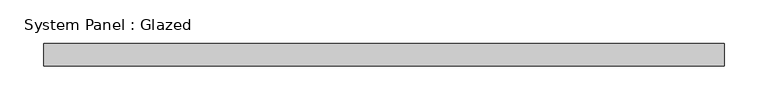
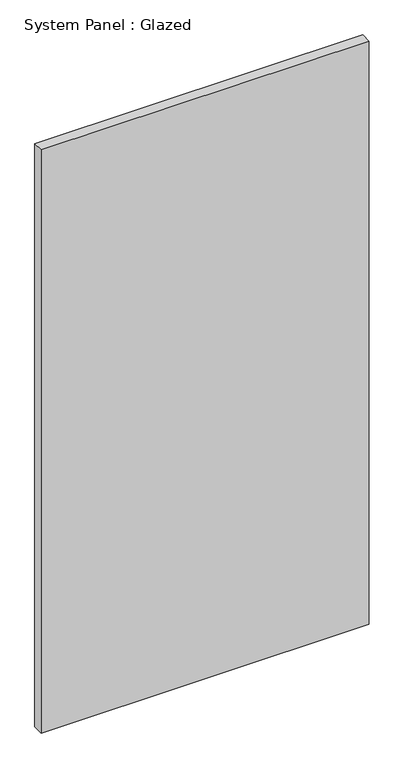
"""IFC4 building model written with IfcOpenShell, lengths in millimetres: plate geometry, System Panel : Glazed."""

from ifc_helpers import new_model, si_unit, origin, origin_with_axes, place, context, project, spatial, polyline, outline, extrude, source, transform, mapped, element, save


def system_panel_glazed_33e8df04(model_context):
    return source(origin(), model_context, "Body", "SweptSolid", [
        extrude(outline(polyline([(388.6438551, 19.05), (-388.6438551, 19.05), (-388.6438551, 44.45), (388.6438551, 44.45), (388.6438551, 19.05)])), origin_with_axes(), (0.0, 0.0, 1.0), 1460.5291864),
    ])


if __name__ == "__main__":
    model = new_model("IFC4")
    model_context = context("Model", 3, world=origin())
    ifc_project = project(units=[si_unit("LENGTHUNIT", "METRE", prefix="MILLI")], contexts=[model_context])
    site = spatial("IfcSite", under=ifc_project)
    building = spatial("IfcBuilding", under=site)
    placement = place(None, origin())
    system_panel_glazed_shape = system_panel_glazed_33e8df04(model_context)
    element("IfcPlate", 1, ObjectType="System Panel : Glazed", at=placement, inside=building, context=model_context, shape_type="MappedRepresentation", body=[
        mapped(system_panel_glazed_shape, transform((0.0, 0.0, 0.0), x_axis=(1.0, 0.0, 0.0), y_axis=(0.0, 1.0, 0.0), z_axis=(0.0, 0.0, 1.0))),
    ])
    save(model, "model.ifc")

# Revit data of these elements
# Type "System Panel : Glazed"
#   Construction Type Id = "GSP4R"
#   Analytic Construction = "1/8 in Pilkington single glazing"
#   Visual Light Transmittance = 0.9
#   Solar Heat Gain Coefficient = 0.86
#   Heat Transfer Coefficient (U) = 1.18115 BTU/(h·ft²·°F)
#   Define Thermal Properties by = 1
# Element 1 (IfcPlate, "System Panel : Glazed")
#   Materials on its faces: "Glass"
# Materials
#   "Glass": class "Glass", colour RGB 0 128 192, transparency 0.75, Description = "Soda Lime Glass", Cost = 0
